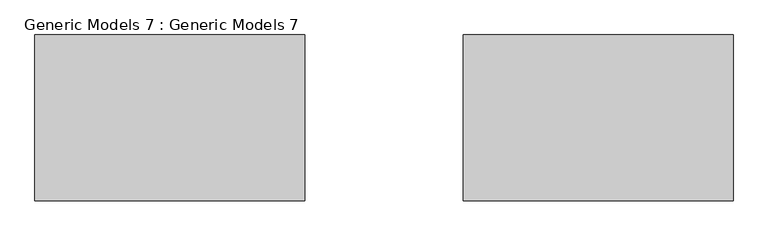
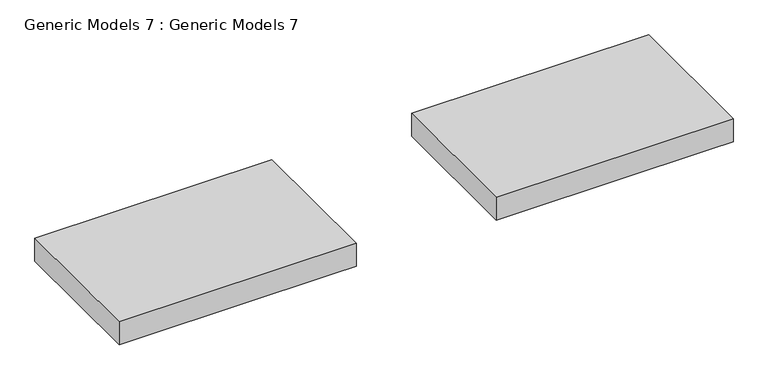
"""IFC4 building model written with IfcOpenShell, lengths in millimetres: proxy geometry, Generic Models 7 : Generic Models 7."""

from ifc_helpers import new_model, si_unit, frame, origin, place, context, project, spatial, polyline, outline, extrude, source, transform, mapped, element, save


def generic_models_7_generic_models_7_55042171(model_context):
    return source(origin(), model_context, "Body", "SweptSolid", [
        extrude(outline(polyline([(2190.75, -36872.9645004), (2190.75, -36720.5645004), (2190.75, -35539.4645004), (2190.75, -35387.0645004), (2343.15, -35387.0645004), (2343.15, -36872.9645004), (2190.75, -36872.9645004)])), frame((0.0, 19682.7756148, 0.0), z_axis=(0.0, 1.0, 0.0), x_axis=(0.0, 0.0, 1.0)), (0.0, 0.0, 1.0), 914.4),
        extrude(outline(polyline([(2190.75, -34510.7645004), (2190.75, -34358.3645004), (2190.75, -33177.2645004), (2190.75, -33024.8645004), (2343.15, -33024.8645004), (2343.15, -34510.7645004), (2190.75, -34510.7645004)])), frame((0.0, 19682.7756148, 0.0), z_axis=(0.0, 1.0, 0.0), x_axis=(0.0, 0.0, 1.0)), (0.0, 0.0, 1.0), 914.4),
    ])


if __name__ == "__main__":
    model = new_model("IFC4")
    model_context = context("Model", 3, world=origin())
    ifc_project = project(units=[si_unit("LENGTHUNIT", "METRE", prefix="MILLI")], contexts=[model_context])
    site = spatial("IfcSite", under=ifc_project)
    building = spatial("IfcBuilding", under=site)
    placement = place(None, origin())
    generic_models_7_generic_models_7_shape = generic_models_7_generic_models_7_55042171(model_context)
    element("IfcBuildingElementProxy", 1, Name="Generic Models 7 : Generic Models 7", ObjectType="Generic Models 7 : Generic Models 7", at=placement, inside=building, context=model_context, shape_type="MappedRepresentation", body=[
        mapped(generic_models_7_generic_models_7_shape, transform((0.0, 0.0, 0.0), x_axis=(1.0, 0.0, 0.0), y_axis=(0.0, 1.0, 0.0), z_axis=(0.0, 0.0, 1.0))),
    ])
    save(model, "model.ifc")
